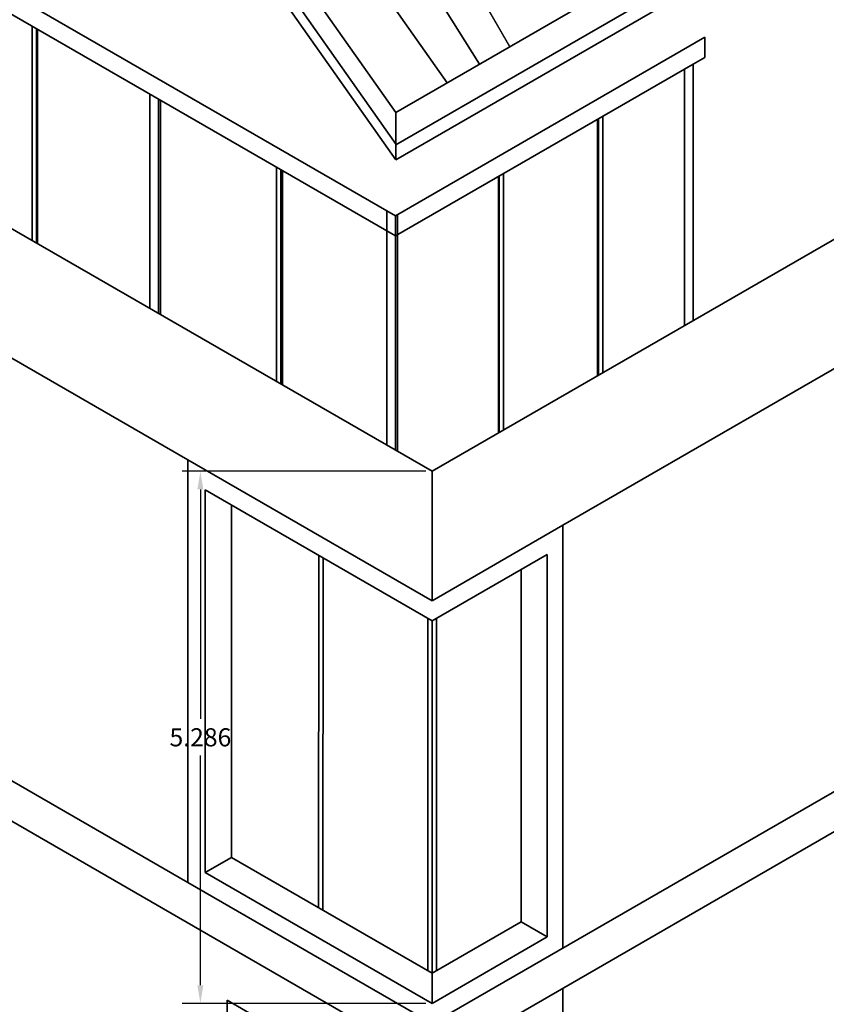
# Model space of a CAD drawing. Units: metres. Extents: x 12735 to 25554, y 20954 to 41989.
# Tile 12 of 15: x 12756 to 12764, y 20971 to 20981. Entities that reach past the tile are written whole.
import ezdxf

# ---------------------------------------------------------------- set-up
doc = ezdxf.new("R2010")
doc.units = ezdxf.units.M
doc.layers.get('Defpoints').update_dxf_attribs({"lineweight": 13})
for name, color, linetype, lineweight in [('A-ANNO-DIMS', 2, 'Continuous', 18), ('A-ELEV', 7, 'Continuous', 35), ('A-ROOF', 1, 'Continuous', 25)]:
    doc.layers.add(name, color=color, linetype=linetype, lineweight=lineweight)
doc.styles.get("Standard").update_dxf_attribs({"font": 'arial.ttf'})
doc.dimstyles.get("Standard").update_dxf_attribs({"dimtxt": 0.18, "dimasz": 0.18, "dimexe": 0.18, "dimexo": 0.0625, "dimgap": 0.09, "dimtad": 0, "dimtih": 1, "dimtoh": 1, "dimdec": 4, "dimzin": 0, "dimdsep": 46, "dimtxsty": 'Standard', "dimcen": 0.09, "dimadec": 0, "dimazin": 0, "dimtfac": 1, "dimtdec": 4, "dimtofl": 0, "dimtmove": 0, "dimatfit": 3, "dimfxl": 1, "dimtolj": 1, "dimtzin": 0, "dimarcsym": 0})

# ---------------------------------------------------------------- blocks, each defined once
blk = doc.blocks.new('*D10')
at = {"layer": 'A-ANNO-DIMS', "color": 0, "lineweight": -2, "transparency": 16777216}
for p, q in [((12766.6445, 20994.8247), (12783.4841, 20994.8247)), ((12783.3041, 20994.6447), (12783.3041, 20975.781)), ((12783.3041, 20956.5534), (12783.3041, 20975.4171)), ((12755.8494, 20956.3734), (12783.4841, 20956.3734))]:
    blk.add_line(p, q, dxfattribs=at)
at = {"layer": 'A-ANNO-DIMS', "color": 0, "transparency": 16777216}
for points in [[(12783.2741, 20994.6447), (12783.3341, 20994.6447), (12783.3041, 20994.8247)], [(12783.2741, 20956.5534), (12783.3341, 20956.5534), (12783.3041, 20956.3734)]]:
    blk.add_solid(points, dxfattribs=at)
at = {"layer": 'Defpoints', "color": 0, "transparency": 16777216}
for p in [(12766.582, 20994.8247), (12783.3041, 20994.8247), (12755.7869, 20956.3734)]:
    blk.add_point(p, dxfattribs=at)
at = {"layer": 'A-ANNO-DIMS', "color": 0, "transparency": 16777216, "insert": (12783.3041, 20975.599), "char_height": 0.18, "attachment_point": 5}
blk.add_mtext('\\A1;38.45', dxfattribs=at)
blk = doc.blocks.new('*D14')
at = {"layer": 'A-ANNO-DIMS', "color": 0, "lineweight": -2, "transparency": 16777216}
for p, q in [((12766.6995, 20994.8564), (12783.4841, 20994.8564)), ((12783.3041, 20994.6764), (12783.3041, 20980.9019)), ((12783.3041, 20966.7635), (12783.3041, 20980.538)), ((12760.5894, 20966.5835), (12783.4841, 20966.5835))]:
    blk.add_line(p, q, dxfattribs=at)
at = {"layer": 'A-ANNO-DIMS', "color": 0, "transparency": 16777216}
for points in [[(12783.2741, 20994.6764), (12783.3341, 20994.6764), (12783.3041, 20994.8564)], [(12783.2741, 20966.7635), (12783.3341, 20966.7635), (12783.3041, 20966.5835)]]:
    blk.add_solid(points, dxfattribs=at)
at = {"layer": 'Defpoints', "color": 0, "transparency": 16777216}
for p in [(12766.637, 20994.8564), (12783.3041, 20994.8564), (12760.5269, 20966.5835)]:
    blk.add_point(p, dxfattribs=at)
at = {"layer": 'A-ANNO-DIMS', "color": 0, "transparency": 16777216, "insert": (12783.3041, 20980.72), "char_height": 0.18, "attachment_point": 5}
blk.add_mtext('\\A1;28.273', dxfattribs=at)
blk = doc.blocks.new('*D16')
at = {"layer": 'A-ANNO-DIMS', "color": 0, "lineweight": -2, "transparency": 16777216}
for p, q in [((12760.1662, 20976.3473), (12757.7487, 20976.3473)), ((12757.9287, 20976.1673), (12757.9287, 20973.8862)), ((12757.9287, 20971.2413), (12757.9287, 20973.5224)), ((12760.1662, 20971.0613), (12757.7487, 20971.0613))]:
    blk.add_line(p, q, dxfattribs=at)
at = {"layer": 'A-ANNO-DIMS', "color": 0, "transparency": 16777216}
for points in [[(12757.8987, 20976.1673), (12757.9587, 20976.1673), (12757.9287, 20976.3473)], [(12757.8987, 20971.2413), (12757.9587, 20971.2413), (12757.9287, 20971.0613)]]:
    blk.add_solid(points, dxfattribs=at)
at = {"layer": 'Defpoints', "color": 0, "transparency": 16777216}
for p in [(12757.9287, 20976.3473), (12760.2287, 20976.3473), (12760.2287, 20971.0613)]:
    blk.add_point(p, dxfattribs=at)
at = {"layer": 'A-ANNO-DIMS', "color": 0, "transparency": 16777216, "insert": (12757.9287, 20973.7043), "char_height": 0.18, "attachment_point": 5}
blk.add_mtext('\\A1;5.286', dxfattribs=at)
blk = doc.blocks.new('*D19')
at = {"layer": 'A-ANNO-DIMS', "color": 0, "lineweight": -2, "transparency": 16777216}
for p, q in [((12747.3297, 20976.0788), (12747.3297, 20997.3364)), ((12773.3057, 20974.7738), (12773.3057, 20997.3364)), ((12747.5097, 20997.1564), (12759.8526, 20997.1564)), ((12773.1257, 20997.1564), (12760.7828, 20997.1564))]:
    blk.add_line(p, q, dxfattribs=at)
at = {"layer": 'A-ANNO-DIMS', "color": 0, "transparency": 16777216}
for points in [[(12747.5097, 20997.1864), (12747.5097, 20997.1264), (12747.3297, 20997.1564)], [(12773.1257, 20997.1864), (12773.1257, 20997.1264), (12773.3057, 20997.1564)]]:
    blk.add_solid(points, dxfattribs=at)
at = {"layer": 'Defpoints', "color": 0, "transparency": 16777216}
for p in [(12773.3057, 20997.1564), (12747.3297, 20976.0163), (12773.3057, 20974.7113)]:
    blk.add_point(p, dxfattribs=at)
at = {"layer": 'A-ANNO-DIMS', "color": 0, "transparency": 16777216, "insert": (12760.3177, 20997.1564), "char_height": 0.18, "attachment_point": 5}
blk.add_mtext('\\A1;25.976', dxfattribs=at)

msp = doc.modelspace()

# ---------------------------------------------------------------- linework, layer by layer
at = {"layer": 'A-ELEV'}
for p, q in [((12760.6982, 20980.3905), (12755.6472, 20988.5115)), ((12754.8551, 20988.0542), (12760.3792, 20980.2064)), ((12754.3454, 20987.7599), (12759.8695, 20979.9121)), ((12754.3454, 20987.4453), (12759.8725, 20979.5932)), ((12754.3454, 20987.2893), (12759.8695, 20979.4415)), ((12759.8695, 20979.9121), (12771.4162, 20986.5786)), ((12759.8695, 20979.5915), (12771.4162, 20986.258)), ((12759.8695, 20979.4415), (12771.3526, 20986.0713)), ((12755.3743, 20981.4792), (12759.8671, 20978.8853)), ((12755.3743, 20981.2792), (12759.8671, 20978.6853)), ((12756.2579, 20980.7691), (12756.2579, 20978.6399)), ((12756.3012, 20980.7441), (12756.3012, 20978.6149)), ((12756.3098, 20980.7391), (12756.3098, 20978.6099)), ((12759.8671, 20978.8853), (12762.9383, 20980.6585)), ((12762.9383, 20980.4585), (12762.9383, 20980.6585)), ((12759.8671, 20978.6853), (12762.8221, 20980.3914)), ((12762.8221, 20980.3914), (12762.9383, 20980.4585)), ((12762.8221, 20980.3914), (12762.8221, 20977.8446)), ((12762.7355, 20980.3414), (12762.7355, 20977.7946)), ((12757.427, 20980.0941), (12757.427, 20977.9649)), ((12757.5136, 20980.0441), (12757.5136, 20977.9149)), ((12757.5309, 20980.0341), (12757.5309, 20977.9049)), ((12759.8695, 20979.4415), (12759.8695, 20979.9121)), ((12761.8717, 20979.8427), (12761.8717, 20977.2959)), ((12761.8804, 20979.8477), (12761.8804, 20977.3009)), ((12761.9237, 20979.8727), (12761.9237, 20977.3259)), ((12765.9791, 20979.6673), (12760.2287, 20976.3473)), ((12758.6827, 20979.3691), (12758.6827, 20977.2399)), ((12758.726, 20979.3441), (12758.726, 20977.2149)), ((12758.7434, 20979.3341), (12758.7434, 20977.2049)), ((12760.8867, 20979.274), (12760.8867, 20976.7272)), ((12760.8954, 20979.279), (12760.8954, 20976.7322)), ((12760.9387, 20979.304), (12760.9387, 20976.7572)), ((12760.2287, 20976.3473), (12755.379, 20979.1473)), ((12759.7805, 20978.9353), (12759.7805, 20976.6061)), ((12759.8671, 20978.8853), (12759.8671, 20976.5561)), ((12759.8844, 20978.8953), (12759.8844, 20976.5461)), ((12756.3012, 20978.6665), (12756.3098, 20978.6715)), ((12761.5277, 20975.8113), (12765.9783, 20978.3809)), ((12757.8038, 20976.4613), (12755.379, 20977.8613)), ((12761.8804, 20977.3009), (12761.8717, 20977.3059)), ((12760.8954, 20976.7322), (12760.8867, 20976.7372)), ((12760.2287, 20975.0613), (12757.8038, 20976.4613)), ((12757.8038, 20976.4613), (12757.8038, 20972.2613)), ((12760.2287, 20975.0613), (12760.2287, 20976.3473)), ((12760.2287, 20974.8613), (12757.977, 20976.1613)), ((12757.977, 20976.1613), (12757.977, 20972.3613)), ((12758.2368, 20976.0113), (12758.2368, 20972.5113)), ((12760.2287, 20975.0613), (12761.5277, 20975.8113)), ((12760.2287, 20975.0613), (12761.5277, 20975.8113)), ((12761.5277, 20975.8113), (12761.5277, 20971.6113)), ((12761.5277, 20971.6113), (12761.5277, 20975.6373)), ((12759.1029, 20975.5113), (12759.102, 20972.0118)), ((12760.2287, 20974.8613), (12761.3724, 20975.5217)), ((12761.3724, 20975.5217), (12761.3724, 20971.7217)), ((12759.1462, 20975.4863), (12759.1453, 20971.9868)), ((12761.1126, 20975.3717), (12761.1126, 20971.8717)), ((12760.1854, 20971.3863), (12760.1854, 20974.8863)), ((12760.2287, 20971.0613), (12760.2287, 20974.8613)), ((12760.272, 20971.3863), (12760.272, 20974.8863)), ((12760.2287, 20970.8613), (12766.174, 20974.2939)), ((12760.2287, 20970.4613), (12766.174, 20973.8939)), ((12757.8038, 20972.2613), (12755.379, 20973.6613)), ((12760.2287, 20970.4613), (12755.379, 20973.2613)), ((12757.977, 20972.3613), (12758.2368, 20972.5113)), ((12760.2287, 20971.3613), (12758.2368, 20972.5113)), ((12757.977, 20972.3613), (12760.2287, 20971.0613)), ((12757.8038, 20972.2613), (12760.2287, 20970.8613)), ((12761.1126, 20971.8717), (12760.2287, 20971.3613)), ((12761.3724, 20971.7217), (12761.1126, 20971.8717)), ((12760.2287, 20971.0613), (12761.3724, 20971.7217)), ((12761.5277, 20967.9113), (12761.5277, 20971.2113)), ((12758.1953, 20971.0921), (12760.1797, 20969.9464)), ((12758.1953, 20969.4259), (12758.1953, 20971.0921))]:
    msp.add_line(p, q, dxfattribs=at)
at = {"layer": 'A-ROOF'}
msp.add_line((12761.0019, 20980.5659), (12756.2227, 20988.8437), dxfattribs=at)
at = {"layer": 'Defpoints'}
msp.add_point((12760.8521, 20979.254), dxfattribs=at)

# ---------------------------------------------------------------- dimensions: what is measured, and where the dimension line sits
at = {"layer": 'A-ANNO-DIMS'}
dim = msp.add_linear_dim(base=(12773.3057, 20997.1564), p1=(12747.3297, 20976.0163), p2=(12773.3057, 20974.7113), dimstyle='Standard', override={"dimdec": 3, "dimlfac": 1, "dimrnd": 0, "dimzin": 0, "dimdsep": 46, "dimlunit": 2}, dxfattribs=at)
dim.commit()
dim.dimension.update_dxf_attribs({"geometry": '*D19', "text_midpoint": (12760.3177, 20997.1564)})
for base, p1, p2, override, picture, middle in [((12783.3041, 20994.8247), (12755.7869, 20956.3734), (12766.582, 20994.8247), {"dimdec": 2, "dimlfac": 1, "dimrnd": 0, "dimzin": 0, "dimdsep": 46, "dimlunit": 2}, '*D10', (12783.3041, 20975.599)), ((12783.3041, 20994.8564), (12760.5269, 20966.5835), (12766.637, 20994.8564), {"dimdec": 3, "dimlfac": 1, "dimrnd": 0, "dimzin": 0, "dimdsep": 46, "dimlunit": 2}, '*D14', (12783.3041, 20980.72)), ((12757.9287, 20976.3473), (12760.2287, 20971.0613), (12760.2287, 20976.3473), {"dimdec": 3, "dimlfac": 1, "dimrnd": 0, "dimzin": 0, "dimdsep": 46, "dimlunit": 2}, '*D16', (12757.9287, 20973.7043))]:
    dim = msp.add_linear_dim(base=base, p1=p1, p2=p2, angle=90, dimstyle='Standard', override=override, dxfattribs=at)
    dim.commit()
    dim.dimension.update_dxf_attribs({"geometry": picture, "text_midpoint": middle})

doc.saveas('drawing.dxf')
